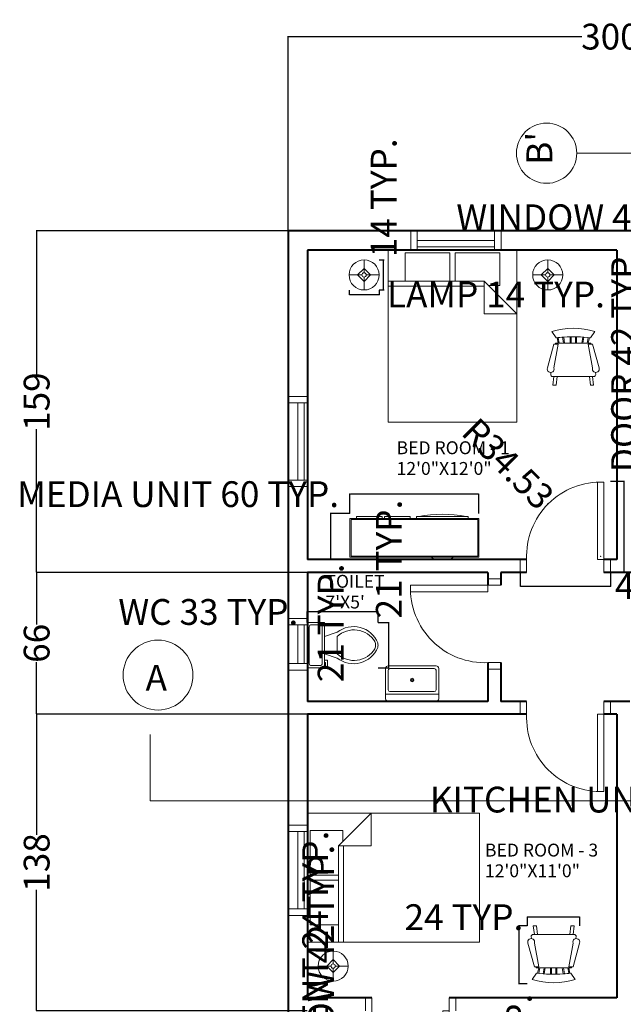
# Model space of a CAD drawing. Units: inches. Extents: x -101 to 786, y 26 to 880.
# Tile 3 of 9: x -101 to 180, y 422 to 880. Entities that reach past the tile are written whole.
import ezdxf

# ---------------------------------------------------------------- set-up
doc = ezdxf.new("R2010")
doc.units = ezdxf.units.IN
doc.header["$MEASUREMENT"] = 0
for name, color, linetype, lineweight in [('A-ANNO-DIMS', 2, 'Continuous', 18), ('A-ANNO-SYMB', 2, 'Continuous', 18), ('A-AREA-IDEN', 7, 'Continuous', 18), ('A-DOOR', 4, 'Continuous', 20), ('A-EQPM', 8, 'Continuous', 13), ('A-FLOR-FIXT', 8, 'Continuous', 18), ('A-FURN', 8, 'Continuous', 13), ('A-GLAZ', 4, 'Continuous', 18), ('A-WALL', 7, 'Continuous', 40)]:
    doc.layers.add(name, color=color, linetype=linetype, lineweight=lineweight)
doc.styles.get("Standard").update_dxf_attribs({"font": 'arial.ttf'})
doc.dimstyles.get("Standard").update_dxf_attribs({"dimtxt": 12, "dimasz": 0.18, "dimexe": 0.18, "dimexo": 0.0625, "dimgap": 0.09, "dimtad": 0, "dimdec": 1, "dimzin": 0, "dimdsep": 46, "dimlunit": 3, "dimtxsty": 'Standard', "dimcen": 0.09, "dimadec": 0, "dimazin": 0, "dimtfac": 1, "dimtdec": 1, "dimtofl": 0, "dimtmove": 0, "dimatfit": 3, "dimfxl": 1, "dimtolj": 1, "dimtzin": 0, "dimarcsym": 0})

# ---------------------------------------------------------------- blocks, each defined once
blk = doc.blocks.new('Bed - Queen')
for p, q in [((0, -80.00003), (0, 0)), ((0, 0), (59.99999, 0)), ((59.99999, 0), (59.99999, -80.00003)), ((7.99999, -1.2), (28.79998, -1.2)), ((7.99999, -14.4), (7.99999, -1.2)), ((28.79998, -1.2), (28.79998, -14.4)), ((31.19999, -1.2), (51.99999, -1.2)), ((31.19999, -14.4), (31.19999, -1.2)), ((51.99999, -1.2), (51.99999, -16.4)), ((0, -14.4), (44.8, -14.4)), ((44.8, -16.8), (0, -16.8)), ((59.99999, -29.6), (44.8, -14.4)), ((44.8, -14.4), (44.8, -29.6)), ((51.99999, -16.4), (46.79936, -16.4)), ((44.8, -29.6), (59.99999, -29.6)), ((59.99999, -80.00003), (0, -80.00003))]:
    blk.add_line(p, q)
blk = doc.blocks.new('Lamp - Table')
for p, q in [((0, 7), (0, 1)), ((-1, 0), (-7, 0)), ((0, 3), (-3, 0)), ((-3, 0), (0, -3)), ((3, 0), (0, 3)), ((0, -3), (3, 0)), ((1, 0), (7, 0)), ((0, -1), (0, -7))]:
    blk.add_line(p, q)
for radius in [7, 1]:
    blk.add_circle((0, 0), radius)
blk = doc.blocks.new('Toilet - top')
for p, q in [((9.5, -6), (9.5, -2)), ((-10, -8.5), (-8, -8.5)), ((-10, -9.5), (-10, -8.5)), ((-8, -8.5), (-8, -8)), ((-7, -8), (-7, -9.5)), ((-4, -8), (-6, -14)), ((4, -8), (6, -14)), ((-7, -9.5), (-10, -9.5)), ((4, -14), (-4, -14))]:
    blk.add_line(p, q)
blk.add_lwpolyline([(10.5, -8), (10.5, 0), (-10.5, 0), (-10.5, -8)], close=True)
for points in [[(-9.5, -2), (-9.5, -6)], [(8.5, -1), (-8.5, -1)], [(-8.5, -7), (8.5, -7)]]:
    blk.add_lwpolyline(points)
for centre, radius, start, end in [((-8.62, -1.88), 0.884, 81.8699, 188.1301), ((8.62, -1.88), 0.884, 351.8699, 98.1301), ((-8.62, -6.12), 0.884, 171.8699, 278.1301), ((8.62, -6.12), 0.884, 261.8699, 8.1301), ((3.52, -21.58), 12.17, 141.4691, 247.9714), ((4.2, -21.82), 11.33, 136.3677, 238.9468), ((-3.52, -21.58), 12.17, 292.0284, 38.5307), ((-4.2, -21.82), 11.33, 301.053, 43.6321), ((0, -27.88), 4, 245.7318, 294.2682), ((0, -29), 4, 254.8605, 285.1395)]:
    blk.add_arc(centre, radius, start, end)
blk = doc.blocks.new('Sink-single - 30 in top')
blk.add_line((-15, -3.999996), (15, -3.999996))
for points in [[(-13.5, 0), (13.5, 0)], [(-15, -18.499996), (-15, -1.5)], [(-12.5, -5.499996), (12.5, -5.499996)], [(15, -1.5), (15, -18.499996)], [(-13.5, -17.499996), (-13.5, -6.499996)], [(13.5, -6.499996), (13.5, -17.499996)], [(13.5, -19.999996), (-13.5, -19.999996)], [(12.5, -18.499996), (-12.5, -18.499996)]]:
    blk.add_lwpolyline(points)
for radius in [1, 0.5]:
    blk.add_circle((0, -11.999996), radius)
for centre, radius, start, end in [((-13.5, -1.5), 1.5, 90, 180), ((-12.5, -6.499996), 1, 90, 180), ((12.5, -6.499996), 1, 0, 90), ((13.5, -1.5), 1.5, 0, 90), ((-13.5, -18.499996), 1.5, 180, 270), ((-12.5, -17.499996), 1, 180, 270), ((12.5, -17.499996), 1, 270, 0), ((13.5, -18.499996), 1.5, 270, 0)]:
    blk.add_arc(centre, radius, start, end)
blk = doc.blocks.new('Entertainment Center')
for p, q in [((-4, 0), (-5, -1)), ((4, 0), (-4, 0)), ((5, -1), (4, 0)), ((-17, -19), (-17, -1)), ((-17, -1), (43, -1)), ((-16.5, -18.5), (-16.5, -1.5)), ((-16.5, -1.5), (42.5, -1.5)), ((42.5, -1.5), (42.5, -18.5)), ((43, -1), (43, -19)), ((43, -19), (-17, -19)), ((42.5, -18.5), (-16.5, -18.5)), ((-12, -20), (-12, -19)), ((12, -20), (-12, -20)), ((12, -19), (12, -20)), ((15, -20), (15, -19)), ((27, -20), (15, -20)), ((27, -19), (27, -20)), ((28, -20), (28, -19)), ((40, -20), (28, -20)), ((40, -19), (40, -20))]:
    blk.add_line(p, q)
blk.add_arc((0, 40), 61, 259.6111, 280.3889)
blk = doc.blocks.new('Chair - Rocking')
for p, q in [((-8, -4.5), (-10, -1.5)), ((-7.5, -4.5), (-7, -7)), ((-6.5, -7), (-7.02225, -4.43)), ((-4.5, -7), (-4.96674, -4.19951)), ((-4, -7), (-4.40532, -4.16272)), ((-1.5, -4.05012), (-1.5, -7)), ((-1, -7), (-1, -4.05012)), ((1, -7), (1, -4.04655)), ((1.5, -4.05012), (1.5, -7)), ((4, -7), (4.40187, -4.18694)), ((4.5, -7), (4.96761, -4.19437)), ((6.5, -7), (7, -4.4057)), ((7.5, -4.5), (7, -7)), ((8, -4.5), (10, -1.5)), ((-9, -7.5), (-12, -18.49999)), ((-7, -7.5), (-9, -7.5)), ((-9, -18.49999), (-7, -7.5)), ((-8.23428, -6.99939), (-8.3093, -7.47958)), ((-8.23041, -7), (8.23915, -7)), ((7, -7.5), (9, -7.5)), ((9, -18.49999), (7, -7.5)), ((8.31071, -7.48854), (8.23449, -7.00073)), ((9, -7.5), (12, -18.49999)), ((-10.36644, -20.64523), (-10.5, -21.49999)), ((-9, -22.49999), (-9.5, -26.49999)), ((0, -22.49999), (-9.5, -22.49999)), ((-8, -26.49999), (-7.5, -22.49999)), ((0, -22.49999), (9.5, -22.49999)), ((8, -26.49999), (7.5, -22.49999)), ((9, -22.49999), (9.5, -26.49999)), ((10.5, -21.49999), (10.3575, -20.58798)), ((-9.5, -26.49999), (-8, -26.49999)), ((9.5, -26.49999), (8, -26.49999))]:
    blk.add_line(p, q)
for centre, radius, start, end in [((0, -34.08333), 34.08333, 72.93847, 107.0615), ((0, -68.25004), 64.25, 93.92211, 97.15267), ((0, -68.25004), 64.25, 82.84733, 93.92211), ((-10.5, -18.99999), 1.58114, 161.5651, 18.43495), ((-9.5, -21.49999), 1, 180, 270), ((10.5, -18.99999), 1.58114, 161.5651, 18.43495), ((9.5, -21.49999), 1, 270, 0)]:
    blk.add_arc(centre, radius, start, end)
blk = doc.blocks.new('DOOR-SINGLE-36')
for p, q in [((-39, 0), (-39, -6)), ((-36, 0), (-36, -6)), ((0, 0), (0, -6)), ((3, 0), (3, -6))]:
    blk.add_line(p, q)
blk.add_lwpolyline([(0, 0), (-3, 0), (-3, 36), (0, 36)], close=True)
blk.add_arc((-1.5, 1.5), 34.53, 87.5104, 182.4896)
blk = doc.blocks.new('WIN-36-WALL9')
for p, q in [((0, 42), (9, 42)), ((0, 39), (9, 39)), ((1.5, 39), (1.5, 3)), ((4.5, 39), (4.5, 3)), ((9, 3), (0, 3)), ((9, 0), (0, 0))]:
    blk.add_line(p, q)
blk = doc.blocks.new('WIN-36-WALL9-FRAMED')
for p, q in [((0, 42), (9, 42)), ((0, 3), (0, 39)), ((0, 39), (9, 39)), ((4.5, 3), (4.5, 39)), ((7.5, 3), (7.5, 39)), ((9, 39), (9, 3)), ((9, 3), (0, 3)), ((9, 0), (0, 0))]:
    blk.add_line(p, q)
blk = doc.blocks.new('VENT-18-WALL9')
for p, q in [((9, 24), (0, 24)), ((9, 21), (0, 21)), ((4.5, 3), (4.5, 21)), ((7.5, 3), (7.5, 21)), ((0, 3), (9, 3)), ((0, 0), (9, 0))]:
    blk.add_line(p, q)
blk = doc.blocks.new('*D31')
at = {"layer": 'A-ANNO-DIMS', "color": 0, "lineweight": -2, "transparency": 16777216}
for p, q in [((134.84, 458.3), (130.68, 458.3)), ((130.86, 458.12), (130.86, 431.48)), ((134.84, 431.3), (130.68, 431.3)), ((130.86, 431.3), (130.86, 431.12))]:
    blk.add_line(p, q, dxfattribs=at)
at = {"layer": 'A-ANNO-DIMS', "color": 0, "transparency": 16777216}
for points in [[(130.83, 458.12), (130.89, 458.12), (130.86, 458.3)], [(130.83, 431.48), (130.89, 431.48), (130.86, 431.3)]]:
    blk.add_solid(points, dxfattribs=at)
at = {"layer": 'Defpoints', "color": 0, "transparency": 16777216}
for p in [(134.91, 458.3), (130.86, 431.3), (134.91, 431.3)]:
    blk.add_point(p, dxfattribs=at)
at = {"layer": 'A-ANNO-DIMS', "color": 0, "transparency": 16777216, "insert": (130.86, 373.49), "char_height": 12, "attachment_point": 5, "rotation": 90}
blk.add_mtext('\\A1;CHAIR 27 TYP.', dxfattribs=at)
blk = doc.blocks.new('*D32')
at = {"layer": 'A-ANNO-DIMS', "color": 0, "lineweight": -2, "transparency": 16777216}
for p, q in [((134.91, 462.35), (134.73, 462.35)), ((134.91, 458.37), (134.91, 462.53)), ((159.16, 462.35), (135.09, 462.35)), ((159.34, 458.37), (159.34, 462.53))]:
    blk.add_line(p, q, dxfattribs=at)
at = {"layer": 'A-ANNO-DIMS', "color": 0, "transparency": 16777216}
for points in [[(135.09, 462.38), (135.09, 462.32), (134.91, 462.35)], [(159.16, 462.38), (159.16, 462.32), (159.34, 462.35)]]:
    blk.add_solid(points, dxfattribs=at)
at = {"layer": 'Defpoints', "color": 0, "transparency": 16777216}
for p in [(134.91, 462.35), (134.91, 458.3), (159.34, 458.3)]:
    blk.add_point(p, dxfattribs=at)
at = {"layer": 'A-ANNO-DIMS', "color": 0, "transparency": 16777216, "insert": (105.33, 462.35), "char_height": 12, "attachment_point": 5, "rotation": 0}
blk.add_mtext('\\A1;24 TYP.', dxfattribs=at)
blk = doc.blocks.new('*D35')
at = {"layer": 'A-ANNO-DIMS', "color": 0, "lineweight": -2, "transparency": 16777216}
for p, q in [((173.57, 665.22), (180.05, 665.22)), ((179.87, 665.22), (179.87, 665.4)), ((179.87, 622.98), (179.87, 665.04)), ((173.57, 622.8), (180.05, 622.8))]:
    blk.add_line(p, q, dxfattribs=at)
at = {"layer": 'A-ANNO-DIMS', "color": 0, "transparency": 16777216}
for points in [[(179.84, 665.04), (179.9, 665.04), (179.87, 665.22)], [(179.84, 622.98), (179.9, 622.98), (179.87, 622.8)]]:
    blk.add_solid(points, dxfattribs=at)
at = {"layer": 'Defpoints', "color": 0, "transparency": 16777216}
for p in [(173.51, 665.22), (179.87, 665.22), (173.51, 622.8)]:
    blk.add_point(p, dxfattribs=at)
at = {"layer": 'A-ANNO-DIMS', "color": 0, "transparency": 16777216, "insert": (179.87, 721.88), "char_height": 12, "attachment_point": 5, "rotation": 90}
blk.add_mtext('\\A1;DOOR 42 TYP.', dxfattribs=at)
blk = doc.blocks.new('*D36')
at = {"layer": 'A-ANNO-DIMS', "color": 0, "lineweight": -2, "transparency": 16777216}
for p, q in [((131.51, 622.74), (131.51, 616.26)), ((173.51, 622.74), (173.51, 616.26)), ((131.69, 616.44), (173.33, 616.44)), ((173.51, 616.44), (173.69, 616.44))]:
    blk.add_line(p, q, dxfattribs=at)
at = {"layer": 'A-ANNO-DIMS', "color": 0, "transparency": 16777216}
for points in [[(131.69, 616.47), (131.69, 616.41), (131.51, 616.44)], [(173.33, 616.47), (173.33, 616.41), (173.51, 616.44)]]:
    blk.add_solid(points, dxfattribs=at)
at = {"layer": 'Defpoints', "color": 0, "transparency": 16777216}
for p in [(131.51, 622.8), (173.51, 622.8), (173.51, 616.44)]:
    blk.add_point(p, dxfattribs=at)
at = {"layer": 'A-ANNO-DIMS', "color": 0, "transparency": 16777216, "insert": (203.22, 616.44), "char_height": 12, "attachment_point": 5}
blk.add_mtext('\\A1;42 TYP.', dxfattribs=at)
blk = doc.blocks.new('*D37')
at = {"layer": 'A-ANNO-DIMS', "color": 0, "lineweight": -2, "transparency": 16777216}
for p, q in [((234.49, 781.87), (234.49, 788.28)), ((276.49, 781.87), (276.49, 788.28)), ((234.49, 788.1), (234.31, 788.1)), ((276.31, 788.1), (234.67, 788.1))]:
    blk.add_line(p, q, dxfattribs=at)
at = {"layer": 'A-ANNO-DIMS', "color": 0, "transparency": 16777216}
for points in [[(234.67, 788.13), (234.67, 788.07), (234.49, 788.1)], [(276.31, 788.13), (276.31, 788.07), (276.49, 788.1)]]:
    blk.add_solid(points, dxfattribs=at)
at = {"layer": 'Defpoints', "color": 0, "transparency": 16777216}
for p in [(234.49, 788.1), (234.49, 781.8), (276.49, 781.8)]:
    blk.add_point(p, dxfattribs=at)
at = {"layer": 'A-ANNO-DIMS', "color": 0, "transparency": 16777216, "insert": (165.66, 788.1), "char_height": 12, "attachment_point": 5}
blk.add_mtext('\\A1;WINDOW 42 TYP.', dxfattribs=at)
blk = doc.blocks.new('*D39')
at = {"layer": 'A-ANNO-DIMS', "color": 0, "lineweight": -2, "transparency": 16777216}
for p, q in [((51.88, 754.19), (51.88, 751.97)), ((52.06, 752.15), (65.7, 752.15)), ((65.88, 754.19), (65.88, 751.97)), ((65.88, 752.15), (66.06, 752.15))]:
    blk.add_line(p, q, dxfattribs=at)
at = {"layer": 'A-ANNO-DIMS', "color": 0, "transparency": 16777216}
for points in [[(52.06, 752.18), (52.06, 752.12), (51.88, 752.15)], [(65.7, 752.18), (65.7, 752.12), (65.88, 752.15)]]:
    blk.add_solid(points, dxfattribs=at)
at = {"layer": 'Defpoints', "color": 0, "transparency": 16777216}
for p in [(51.88, 754.25), (65.88, 754.25), (65.88, 752.15)]:
    blk.add_point(p, dxfattribs=at)
at = {"layer": 'A-ANNO-DIMS', "color": 0, "transparency": 16777216, "insert": (120.24, 752.15), "char_height": 12, "attachment_point": 5}
blk.add_mtext('\\A1;LAMP 14 TYP.', dxfattribs=at)
blk = doc.blocks.new('*D40')
at = {"layer": 'A-ANNO-DIMS', "color": 0, "lineweight": -2, "transparency": 16777216}
for p, q in [((65.94, 768.25), (68.16, 768.25)), ((67.98, 768.25), (67.98, 768.43)), ((67.98, 754.43), (67.98, 768.07)), ((65.94, 754.25), (68.16, 754.25))]:
    blk.add_line(p, q, dxfattribs=at)
at = {"layer": 'A-ANNO-DIMS', "color": 0, "transparency": 16777216}
for points in [[(67.95, 768.07), (68.01, 768.07), (67.98, 768.25)], [(67.95, 754.43), (68.01, 754.43), (67.98, 754.25)]]:
    blk.add_solid(points, dxfattribs=at)
at = {"layer": 'Defpoints', "color": 0, "transparency": 16777216}
for p in [(65.88, 768.25), (67.98, 768.25), (65.88, 754.25)]:
    blk.add_point(p, dxfattribs=at)
at = {"layer": 'A-ANNO-DIMS', "color": 0, "transparency": 16777216, "insert": (67.98, 797.16), "char_height": 12, "attachment_point": 5, "rotation": 90}
blk.add_mtext('\\A1;14 TYP.', dxfattribs=at)
blk = doc.blocks.new('*D49')
at = {"layer": 'A-ANNO-DIMS', "color": 0, "lineweight": -2, "transparency": 16777216}
for p, q in [((32.38, 604.4), (32.2, 604.4)), ((32.38, 599.51), (32.38, 604.58)), ((65.24, 604.4), (32.56, 604.4)), ((65.42, 599.51), (65.42, 604.58))]:
    blk.add_line(p, q, dxfattribs=at)
at = {"layer": 'A-ANNO-DIMS', "color": 0, "transparency": 16777216}
for points in [[(32.56, 604.43), (32.56, 604.37), (32.38, 604.4)], [(65.24, 604.43), (65.24, 604.37), (65.42, 604.4)]]:
    blk.add_solid(points, dxfattribs=at)
at = {"layer": 'Defpoints', "color": 0, "transparency": 16777216}
for p in [(32.38, 604.4), (32.38, 599.45), (65.42, 599.45)]:
    blk.add_point(p, dxfattribs=at)
at = {"layer": 'A-ANNO-DIMS', "color": 0, "transparency": 16777216, "insert": (-13.64, 604.4), "char_height": 12, "attachment_point": 5}
blk.add_mtext('\\A1;WC 33 TYP.', dxfattribs=at)
blk = doc.blocks.new('*D50')
at = {"layer": 'A-ANNO-DIMS', "color": 0, "lineweight": -2, "transparency": 16777216}
for p, q in [((65.48, 599.45), (70.56, 599.45)), ((70.38, 599.45), (70.38, 599.63)), ((70.38, 578.63), (70.38, 599.27)), ((65.48, 578.45), (70.56, 578.45))]:
    blk.add_line(p, q, dxfattribs=at)
at = {"layer": 'A-ANNO-DIMS', "color": 0, "transparency": 16777216}
for points in [[(70.35, 599.27), (70.41, 599.27), (70.38, 599.45)], [(70.35, 578.63), (70.41, 578.63), (70.38, 578.45)]]:
    blk.add_solid(points, dxfattribs=at)
at = {"layer": 'Defpoints', "color": 0, "transparency": 16777216}
for p in [(65.42, 599.45), (70.38, 599.45), (65.42, 578.45)]:
    blk.add_point(p, dxfattribs=at)
at = {"layer": 'A-ANNO-DIMS', "color": 0, "transparency": 16777216, "insert": (70.38, 629.02), "char_height": 12, "attachment_point": 5, "rotation": 90}
blk.add_mtext('\\A1;21 TYP.', dxfattribs=at)
blk = doc.blocks.new('*D51')
at = {"layer": 'A-ANNO-DIMS', "color": 0, "lineweight": -2, "transparency": 16777216}
for p, q in [((32.57, 292.61), (38.99, 292.61)), ((38.81, 292.61), (38.81, 292.79)), ((38.81, 250.79), (38.81, 292.43)), ((32.57, 250.61), (38.99, 250.61))]:
    blk.add_line(p, q, dxfattribs=at)
at = {"layer": 'A-ANNO-DIMS', "color": 0, "transparency": 16777216}
for points in [[(38.78, 292.43), (38.84, 292.43), (38.81, 292.61)], [(38.78, 250.79), (38.84, 250.79), (38.81, 250.61)]]:
    blk.add_solid(points, dxfattribs=at)
at = {"layer": 'Defpoints', "color": 0, "transparency": 16777216}
for p in [(32.51, 292.61), (38.81, 292.61), (32.51, 250.61)]:
    blk.add_point(p, dxfattribs=at)
at = {"layer": 'A-ANNO-DIMS', "color": 0, "transparency": 16777216, "insert": (38.81, 398.57), "char_height": 12, "attachment_point": 5, "rotation": 90}
blk.add_mtext('\\A1;FRAMED WINDOW 42 TYP.', dxfattribs=at)
blk = doc.blocks.new('*D57')
at = {"layer": 'A-ANNO-DIMS', "color": 0, "lineweight": -2, "transparency": 16777216}
for p, q in [((52.3, 659.23), (52.12, 659.23)), ((52.3, 650.29), (52.3, 659.41)), ((112.12, 659.23), (52.48, 659.23)), ((112.3, 650.29), (112.3, 659.41))]:
    blk.add_line(p, q, dxfattribs=at)
at = {"layer": 'A-ANNO-DIMS', "color": 0, "transparency": 16777216}
for points in [[(52.48, 659.26), (52.48, 659.2), (52.3, 659.23)], [(112.12, 659.26), (112.12, 659.2), (112.3, 659.23)]]:
    blk.add_solid(points, dxfattribs=at)
at = {"layer": 'Defpoints', "color": 0, "transparency": 16777216}
for p in [(52.3, 659.23), (52.3, 650.23), (112.3, 650.23)]:
    blk.add_point(p, dxfattribs=at)
at = {"layer": 'A-ANNO-DIMS', "color": 0, "transparency": 16777216, "insert": (-27.66, 659.23), "char_height": 12, "attachment_point": 5}
blk.add_mtext('\\A1;MEDIA UNIT 60 TYP.', dxfattribs=at)
blk = doc.blocks.new('*D58')
at = {"layer": 'A-ANNO-DIMS', "color": 0, "lineweight": -2, "transparency": 16777216}
for p, q in [((52.24, 650.23), (43.12, 650.23)), ((43.3, 650.05), (43.3, 629.08)), ((52.24, 628.9), (43.12, 628.9)), ((43.3, 628.9), (43.3, 628.72))]:
    blk.add_line(p, q, dxfattribs=at)
at = {"layer": 'A-ANNO-DIMS', "color": 0, "transparency": 16777216}
for points in [[(43.27, 650.05), (43.33, 650.05), (43.3, 650.23)], [(43.27, 629.08), (43.33, 629.08), (43.3, 628.9)]]:
    blk.add_solid(points, dxfattribs=at)
at = {"layer": 'Defpoints', "color": 0, "transparency": 16777216}
for p in [(52.3, 650.23), (43.3, 628.9), (52.3, 628.9)]:
    blk.add_point(p, dxfattribs=at)
at = {"layer": 'A-ANNO-DIMS', "color": 0, "transparency": 16777216, "insert": (43.3, 599.32), "char_height": 12, "attachment_point": 5, "rotation": 90}
blk.add_mtext('\\A1;21 TYP.', dxfattribs=at)
blk = doc.blocks.new('*D59')
at = {"layer": 'A-ANNO-DIMS', "color": 0, "lineweight": -2, "transparency": 16777216}
for p, q in [((32.57, 398.32), (36.29, 398.32)), ((36.11, 398.32), (36.11, 398.5)), ((36.11, 374.5), (36.11, 398.14)), ((32.57, 374.32), (36.29, 374.32))]:
    blk.add_line(p, q, dxfattribs=at)
at = {"layer": 'A-ANNO-DIMS', "color": 0, "transparency": 16777216}
for points in [[(36.08, 398.14), (36.14, 398.14), (36.11, 398.32)], [(36.08, 374.5), (36.14, 374.5), (36.11, 374.32)]]:
    blk.add_solid(points, dxfattribs=at)
at = {"layer": 'Defpoints', "color": 0, "transparency": 16777216}
for p in [(32.51, 398.32), (36.11, 398.32), (32.51, 374.32)]:
    blk.add_point(p, dxfattribs=at)
at = {"layer": 'A-ANNO-DIMS', "color": 0, "transparency": 16777216, "insert": (36.11, 452.79), "char_height": 12, "attachment_point": 5, "rotation": 90}
blk.add_mtext('\\A1;VENT 24 TYP.', dxfattribs=at)
blk = doc.blocks.new('*D65')
at = {"layer": 'A-ANNO-DIMS', "color": 0, "lineweight": -2, "transparency": 16777216}
for p, q in [((225.49, 517.07), (225.31, 517.07)), ((225.49, 503.78), (225.49, 517.25)), ((314.33, 517.07), (225.67, 517.07)), ((314.51, 503.78), (314.51, 517.25))]:
    blk.add_line(p, q, dxfattribs=at)
at = {"layer": 'A-ANNO-DIMS', "color": 0, "transparency": 16777216}
for points in [[(225.67, 517.1), (225.67, 517.04), (225.49, 517.07)], [(314.33, 517.1), (314.33, 517.04), (314.51, 517.07)]]:
    blk.add_solid(points, dxfattribs=at)
at = {"layer": 'Defpoints', "color": 0, "transparency": 16777216}
for p in [(225.49, 517.07), (225.49, 503.72), (314.51, 503.72)]:
    blk.add_point(p, dxfattribs=at)
at = {"layer": 'A-ANNO-DIMS', "color": 0, "transparency": 16777216, "insert": (155.88, 517.07), "char_height": 12, "attachment_point": 5}
blk.add_mtext('\\A1;KITCHEN UNIT 89', dxfattribs=at)
blk = doc.blocks.new('*D79')
at = {"layer": 'A-ANNO-DIMS', "color": 0, "lineweight": -2, "transparency": 16777216}
for p, q in [((23.51, 781.87), (23.51, 872.36)), ((23.69, 872.18), (160.19, 872.18)), ((323.33, 872.18), (186.83, 872.18)), ((323.51, 781.87), (323.51, 872.36))]:
    blk.add_line(p, q, dxfattribs=at)
at = {"layer": 'A-ANNO-DIMS', "color": 0, "transparency": 16777216}
for points in [[(23.69, 872.21), (23.69, 872.15), (23.51, 872.18)], [(323.33, 872.21), (323.33, 872.15), (323.51, 872.18)]]:
    blk.add_solid(points, dxfattribs=at)
at = {"layer": 'Defpoints', "color": 0, "transparency": 16777216}
for p in [(323.51, 872.18), (23.51, 781.8), (323.51, 781.8)]:
    blk.add_point(p, dxfattribs=at)
at = {"layer": 'A-ANNO-DIMS', "color": 0, "transparency": 16777216, "insert": (173.51, 872.18), "char_height": 12, "attachment_point": 5}
blk.add_mtext('\\A1;300', dxfattribs=at)
blk = doc.blocks.new('*D83')
at = {"layer": 'A-ANNO-DIMS', "color": 0, "lineweight": -2, "transparency": 16777216}
for p, q in [((32.44, 556.8), (-93.7, 556.8)), ((-93.52, 556.62), (-93.52, 500.6)), ((-93.52, 418.98), (-93.52, 475.01)), ((32.44, 418.8), (-93.7, 418.8))]:
    blk.add_line(p, q, dxfattribs=at)
at = {"layer": 'A-ANNO-DIMS', "color": 0, "transparency": 16777216}
for points in [[(-93.55, 556.62), (-93.49, 556.62), (-93.52, 556.8)], [(-93.55, 418.98), (-93.49, 418.98), (-93.52, 418.8)]]:
    blk.add_solid(points, dxfattribs=at)
at = {"layer": 'Defpoints', "color": 0, "transparency": 16777216}
for p in [(-93.52, 556.8), (32.51, 556.8), (32.51, 418.8)]:
    blk.add_point(p, dxfattribs=at)
at = {"layer": 'A-ANNO-DIMS', "color": 0, "transparency": 16777216, "insert": (-93.52, 487.8), "char_height": 12, "attachment_point": 5, "rotation": 90}
blk.add_mtext('\\A1;138', dxfattribs=at)
blk = doc.blocks.new('*D84')
at = {"layer": 'A-ANNO-DIMS', "color": 0, "lineweight": -2, "transparency": 16777216}
for p, q in [((32.44, 622.8), (-93.7, 622.8)), ((-93.52, 622.62), (-93.52, 598.52)), ((-93.52, 556.98), (-93.52, 581.09)), ((32.44, 556.8), (-93.7, 556.8))]:
    blk.add_line(p, q, dxfattribs=at)
at = {"layer": 'A-ANNO-DIMS', "color": 0, "transparency": 16777216}
for points in [[(-93.55, 622.62), (-93.49, 622.62), (-93.52, 622.8)], [(-93.55, 556.98), (-93.49, 556.98), (-93.52, 556.8)]]:
    blk.add_solid(points, dxfattribs=at)
at = {"layer": 'Defpoints', "color": 0, "transparency": 16777216}
for p in [(-93.52, 622.8), (32.51, 622.8), (32.51, 556.8)]:
    blk.add_point(p, dxfattribs=at)
at = {"layer": 'A-ANNO-DIMS', "color": 0, "transparency": 16777216, "insert": (-93.52, 589.8), "char_height": 12, "attachment_point": 5, "rotation": 90}
blk.add_mtext('\\A1;66', dxfattribs=at)
blk = doc.blocks.new('*D85')
at = {"layer": 'A-ANNO-DIMS', "color": 0, "lineweight": -2, "transparency": 16777216}
for p, q in [((23.44, 781.8), (-93.7, 781.8)), ((-93.52, 781.62), (-93.52, 715.1)), ((-93.52, 622.98), (-93.52, 689.51)), ((32.44, 622.8), (-93.7, 622.8))]:
    blk.add_line(p, q, dxfattribs=at)
at = {"layer": 'A-ANNO-DIMS', "color": 0, "transparency": 16777216}
for points in [[(-93.55, 781.62), (-93.49, 781.62), (-93.52, 781.8)], [(-93.55, 622.98), (-93.49, 622.98), (-93.52, 622.8)]]:
    blk.add_solid(points, dxfattribs=at)
at = {"layer": 'Defpoints', "color": 0, "transparency": 16777216}
for p in [(-93.52, 781.8), (23.51, 781.8), (32.51, 622.8)]:
    blk.add_point(p, dxfattribs=at)
at = {"layer": 'A-ANNO-DIMS', "color": 0, "transparency": 16777216, "insert": (-93.52, 702.3), "char_height": 12, "attachment_point": 5, "rotation": 90}
blk.add_mtext('\\A1;159', dxfattribs=at)
blk = doc.blocks.new('*D129')
at = {"layer": 'A-ANNO-DIMS', "color": 0, "lineweight": -2, "transparency": 16777216}
for p, q in [((144.33, 654.98), (144.46, 654.85)), ((168.92, 630.3), (169.1, 630.3)), ((169.01, 630.21), (169.01, 630.39))]:
    blk.add_line(p, q, dxfattribs=at)
at = {"layer": 'A-ANNO-DIMS', "color": 0, "transparency": 16777216}
blk.add_solid([(144.48, 654.87), (144.44, 654.83), (144.59, 654.72)], dxfattribs=at)
at = {"layer": 'Defpoints', "color": 0, "transparency": 16777216}
for p in [(144.59, 654.72), (169.01, 630.3)]:
    blk.add_point(p, dxfattribs=at)
at = {"layer": 'A-ANNO-DIMS', "color": 0, "transparency": 16777216, "insert": (125.89, 673.42), "char_height": 12, "attachment_point": 5, "rotation": 314.9993}
blk.add_mtext('\\A1;R34.53', dxfattribs=at)

msp = doc.modelspace()

# ---------------------------------------------------------------- linework, layer by layer
at = {"layer": 'A-ANNO-SYMB'}
for p, q in [((183.8117, 817.9238), (157.8207, 817.9238)), ((-40.6288, 516.4544), (-40.6288, 547.4081)), ((-40.6288, 516.4544), (362.9319, 516.4544))]:
    msp.add_line(p, q, dxfattribs=at)
for centre, radius in [((143.8117, 817.9238), 14.0089), ((-37.015, 575.0232), 16.2575)]:
    msp.add_circle(centre, radius, dxfattribs=at)
at = {"layer": 'A-WALL'}
for p, q in [((32.5071, 772.8033), (32.5071, 628.8033)), ((176.5071, 772.8033), (32.5071, 772.8033)), ((176.5071, 772.8033), (176.5071, 628.8033)), ((134.5071, 628.8033), (32.5071, 628.8033)), ((176.5071, 628.8033), (170.5071, 628.8033)), ((32.5071, 622.8033), (32.5071, 562.8033)), ((116.5071, 622.8033), (32.5071, 622.8033)), ((116.5071, 622.8033), (116.5071, 616.8033)), ((122.5071, 622.8033), (122.5071, 616.8033)), ((134.5071, 622.8033), (122.5071, 622.8033)), ((188.5071, 622.8033), (170.5071, 622.8033)), ((116.5071, 580.8033), (116.5071, 562.8033)), ((122.5071, 580.8033), (122.5071, 562.8033)), ((116.5071, 562.8033), (32.5071, 562.8033)), ((134.5071, 562.8033), (122.5071, 562.8033)), ((182.5071, 562.8033), (170.5071, 562.8033)), ((32.5071, 556.8033), (32.5071, 424.8033)), ((134.5071, 556.8033), (32.5071, 556.8033)), ((176.5071, 556.8033), (170.5071, 556.8033)), ((176.5071, 556.8033), (176.5071, 424.8033)), ((62.5071, 424.8033), (32.5071, 424.8033)), ((176.5071, 424.8033), (98.5071, 424.8033))]:
    msp.add_line(p, q, dxfattribs=at)
msp.add_lwpolyline([(323.5071, 151.8033), (323.5071, 781.8033), (23.5071, 781.8033), (23.5071, 151.8033)], dxfattribs=at)

# ---------------------------------------------------------------- block references
at = {"layer": 'A-DOOR'}
msp.add_blockref('DOOR-SINGLE-36', (170.5071, 628.8033), dxfattribs=at)
at = {"layer": 'A-DOOR', "rotation": 89.99999999999957}
msp.add_blockref('DOOR-SINGLE-36', (116.5071, 616.8033), dxfattribs=at)
at = {"layer": 'A-DOOR', "extrusion": (0, 0, -1), "zscale": -1, "rotation": 180}
for p in [(-170.5071, 556.8033), (-98.5071, 418.8033)]:
    msp.add_blockref('DOOR-SINGLE-36', p, dxfattribs=at)
at = {"layer": 'A-EQPM'}
for p in [(58.8794, 761.25), (144.3362, 761.25), (44.4799, 439.5845)]:
    msp.add_blockref('Lamp - Table', p, dxfattribs=at)
at = {"layer": 'A-EQPM', "rotation": 180}
msp.add_blockref('Entertainment Center', (95.3033, 628.896), dxfattribs=at)
at = {"layer": 'A-FLOR-FIXT', "rotation": 90}
msp.add_blockref('Toilet - top', (32.3759, 588.946), dxfattribs=at)
at = {"layer": 'A-FLOR-FIXT', "xscale": 0.8250378517028346, "yscale": 0.8250378517028346, "zscale": 0.8250378517028346, "rotation": 180}
msp.add_blockref('Sink-single - 30 in top', (81.2425, 562.8033), dxfattribs=at)
at = {"layer": 'A-FURN'}
for name, p in [('Bed - Queen', (70.0324, 772.8033)), ('Chair - Rocking', (156.2103, 736.4634))]:
    msp.add_blockref(name, p, dxfattribs=at)
for name, p, rotation in [('Bed - Queen', (32.5071, 450.7571), 90), ('Chair - Rocking', (147.1241, 431.8033), 180.0000007238078)]:
    msp.add_blockref(name, p, dxfattribs=dict(at, rotation=rotation))
at = {"layer": 'A-GLAZ', "rotation": 89.99999999999987}
msp.add_blockref('WIN-36-WALL9', (122.6343, 772.8032), dxfattribs=at)
at = {"layer": 'A-GLAZ'}
for name, p in [('WIN-36-WALL9-FRAMED', (23.507, 662.7466)), ('VENT-18-WALL9', (23.507, 577.3661)), ('WIN-36-WALL9-FRAMED', (23.507, 463.169))]:
    msp.add_blockref(name, p, dxfattribs=at)

# ---------------------------------------------------------------- texts
at = {"layer": 'A-ANNO-SYMB'}
msp.add_text("B'", height=12, rotation=90, dxfattribs=at).set_placement((146.4354, 812.535))
msp.add_text('A', height=12, dxfattribs=at).set_placement((-42.8031, 567.7803))
at = {"layer": 'A-AREA-IDEN'}
for s, p in [('BED ROOM - 1', (73.9827, 677.8288)), ('12\'0"X12\'0"', (73.9827, 668.1903)), ('TOILET', (40.9018, 615.6617)), ("7'X5'", (40.9018, 606.0232)), ('BED ROOM - 3', (115.0942, 490.5631)), ('12\'0"X11\'0"', (115.0942, 480.9246))]:
    msp.add_text(s, height=6, dxfattribs=at).set_placement(p)

# ---------------------------------------------------------------- dimensions: what is measured, and where the dimension line sits
at = {"layer": 'A-ANNO-DIMS'}
dim = msp.add_linear_dim(base=(323.5071, 872.1827), p1=(23.5071, 781.8033), p2=(323.5071, 781.8033), dimstyle='Standard', override={"dimdec": 0, "dimlfac": 1, "dimrnd": 0, "dimzin": 0, "dimdsep": 46, "dimlunit": 2}, dxfattribs=at)
dim.commit()
dim.dimension.update_dxf_attribs({"geometry": '*D79', "text_midpoint": (173.5071, 872.1827)})
for base, p1, p2, angle, text, picture, middle in [((67.9794, 768.25), (65.8794, 754.25), (65.8794, 768.25), 90, '<> TYP.', '*D40', (67.9794, 797.1612)), ((234.4852, 788.1033), (276.4852, 781.8033), (234.4852, 781.8033), 180, 'WINDOW <> TYP.', '*D37', (165.6572, 788.1033)), ((179.8701, 665.2238), (173.5071, 622.8033), (173.5071, 665.2238), 90, 'DOOR <> TYP.', '*D35', (179.8701, 721.8757)), ((52.3033, 659.2293), (112.3033, 650.2293), (52.3033, 650.2293), 180, 'MEDIA UNIT <> TYP.', '*D57', (-27.657, 659.2293)), ((70.3791, 599.446), (65.4222, 578.446), (65.4222, 599.446), 90, '<> TYP.', '*D50', (70.3791, 629.0244)), ((43.3033, 628.896), (52.3033, 650.2293), (52.3033, 628.896), 270, '<> TYP.', '*D58', (43.3033, 599.3177)), ((32.3759, 604.403), (65.4222, 599.446), (32.3759, 599.446), 180, 'WC <> TYP.', '*D49', (-13.639, 604.403)), ((225.4936, 517.0678), (314.5071, 503.7158), (225.4936, 503.7158), 180, 'KITCHEN UNIT <>', '*D65', (155.8798, 517.0678)), ((36.1071, 398.3203), (32.5071, 374.3203), (32.5071, 398.3203), 90, 'VENT <> TYP.', '*D59', (36.1071, 452.7908)), ((38.8071, 292.6111), (32.5071, 250.6111), (32.5071, 292.6111), 90, 'FRAMED WINDOW <> TYP.', '*D51', (38.8071, 398.5728)), ((134.9066, 462.3533), (159.3417, 458.3033), (134.9066, 458.3033), 180.000001, '<> TYP.', '*D32', (105.3283, 462.3533)), ((130.8566, 431.3033), (134.9066, 458.3033), (134.9066, 431.3033), 270.000001, 'CHAIR <> TYP.', '*D31', (130.8566, 373.489))]:
    dim = msp.add_linear_dim(base=base, p1=p1, p2=p2, angle=angle, text=text, dimstyle='Standard', override={"dimdec": 0, "dimlfac": 1, "dimrnd": 0, "dimzin": 0, "dimdsep": 46, "dimlunit": 2}, dxfattribs=at)
    dim.commit()
    dim.dimension.update_dxf_attribs({"geometry": picture, "text_midpoint": middle})
for base, p1, p2, picture, middle in [((-93.5225, 781.8033), (32.5071, 622.8033), (23.5071, 781.8033), '*D85', (-93.5225, 702.3033)), ((-93.5225, 622.8033), (32.5071, 556.8033), (32.5071, 622.8033), '*D84', (-93.5225, 589.8033)), ((-93.5225, 556.8033), (32.5071, 418.8033), (32.5071, 556.8033), '*D83', (-93.5225, 487.8033))]:
    dim = msp.add_linear_dim(base=base, p1=p1, p2=p2, angle=90, dimstyle='Standard', override={"dimdec": 0, "dimlfac": 1, "dimrnd": 0, "dimzin": 0, "dimdsep": 46, "dimlunit": 2}, dxfattribs=at)
    dim.commit()
    dim.dimension.update_dxf_attribs({"geometry": picture, "text_midpoint": middle})
for base, p1, p2, text, picture, middle in [((65.8794, 752.15), (51.8794, 754.25), (65.8794, 754.25), 'LAMP <> TYP.', '*D39', (120.2435, 752.15)), ((173.5071, 616.4402), (131.5071, 622.8033), (173.5071, 622.8033), '<> TYP.', '*D36', (203.2245, 616.4402))]:
    dim = msp.add_linear_dim(base=base, p1=p1, p2=p2, text=text, dimstyle='Standard', override={"dimdec": 0, "dimlfac": 1, "dimrnd": 0, "dimzin": 0, "dimdsep": 46, "dimlunit": 2}, dxfattribs=at)
    dim.commit()
    dim.dimension.update_dxf_attribs({"geometry": picture, "text_midpoint": middle})
dim = msp.add_radius_dim(center=(169.0071, 630.3033), mpoint=(144.5892, 654.7218), dimstyle='Standard', override={"dimdec": 2, "dimlfac": 1, "dimrnd": 0, "dimzin": 0, "dimdsep": 46, "dimlunit": 2}, dxfattribs=at)
dim.commit()
dim.dimension.update_dxf_attribs({"geometry": '*D129', "text_midpoint": (125.8941, 673.4173)})

doc.saveas('drawing.dxf')
